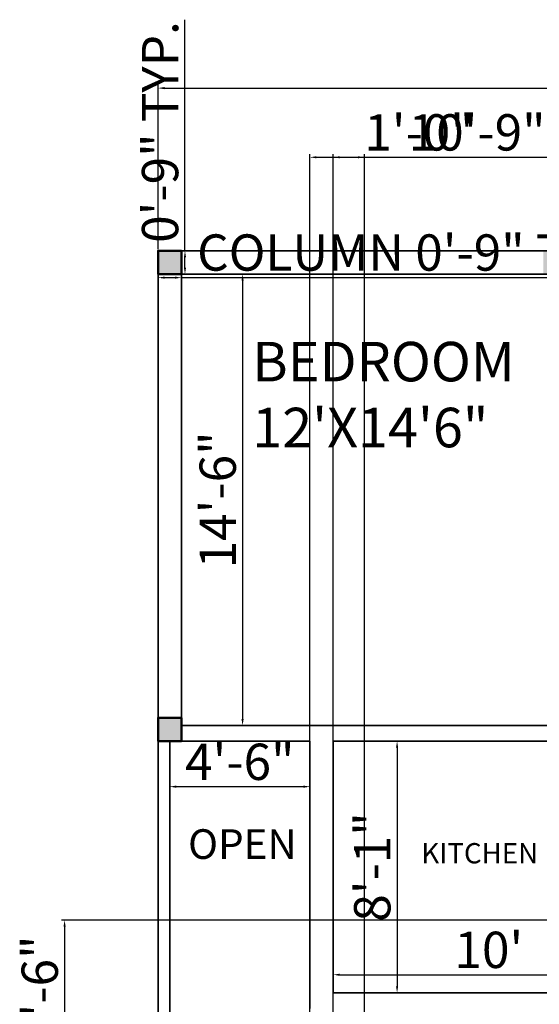
# Model space of a CAD drawing. Units: inches. Extents: x 3316 to 4157, y 2203 to 2977.
# Tile 2 of 4: x 3316 to 3517, y 2597 to 2977. Entities that reach past the tile are written whole.
import ezdxf

# ---------------------------------------------------------------- set-up
doc = ezdxf.new("R2010")
doc.units = ezdxf.units.IN
for name, color, linetype, lineweight in [('A-ANNO-DIMS', 2, 'Continuous', 18), ('A-AREA-IDEN', 7, 'Continuous', 25), ('A-COLS', 7, 'Continuous', 50), ('A-COLS-PATT', 4, 'Continuous', 13), ('A-WALL', 7, 'Continuous', 35), ('C-PROP', 7, 'Continuous', 35)]:
    doc.layers.add(name, color=color, linetype=linetype, lineweight=lineweight)
doc.styles.get("Standard").update_dxf_attribs({"font": 'arial.ttf'})
doc.dimstyles.new('ISO-25', dxfattribs={"dimtxt": 14, "dimasz": 2.5, "dimexe": 1.25, "dimexo": 0.625, "dimtad": 1, "dimlunit": 3, "dimtxsty": 'Standard', "dimcen": 2.5, "dimadec": 0, "dimazin": 0, "dimtfac": 1, "dimtmove": 0, "dimatfit": 3, "dimfxl": 1, "dimarcsym": 0})

# ---------------------------------------------------------------- blocks, each defined once
blk = doc.blocks.new('*D3')
at = {"layer": 'A-ANNO-DIMS', "color": 0, "lineweight": -2, "transparency": 16777216}
for p, q in [((3402.76, 2878.84), (3403.39, 2878.84)), ((3402.14, 2876.34), (3402.14, 2707.34)), ((3402.76, 2704.84), (3403.39, 2704.84))]:
    blk.add_line(p, q, dxfattribs=at)
at = {"layer": 'A-ANNO-DIMS', "color": 0, "transparency": 16777216}
for points in [[(3401.72, 2876.34), (3402.55, 2876.34), (3402.14, 2878.84)], [(3401.72, 2707.34), (3402.55, 2707.34), (3402.14, 2704.84)]]:
    blk.add_solid(points, dxfattribs=at)
at = {"layer": 'Defpoints', "color": 0, "transparency": 16777216}
for p in [(3402.14, 2878.84), (3402.14, 2704.84), (3402.14, 2704.84)]:
    blk.add_point(p, dxfattribs=at)
at = {"layer": 'A-ANNO-DIMS', "color": 0, "transparency": 16777216, "insert": (3394.37, 2791.84), "char_height": 14, "attachment_point": 5, "rotation": 90}
blk.add_mtext('14\'-6"', dxfattribs=at)
blk = doc.blocks.new('*D6')
at = {"layer": 'A-ANNO-DIMS', "color": 0, "lineweight": -2, "transparency": 16777216}
for p, q in [((3369.58, 2888.47), (3369.58, 2951.81)), ((3372.08, 2950.56), (3847.08, 2950.56)), ((3849.58, 2888.47), (3849.58, 2951.81))]:
    blk.add_line(p, q, dxfattribs=at)
at = {"layer": 'A-ANNO-DIMS', "color": 0, "transparency": 16777216}
for points in [[(3372.08, 2950.98), (3372.08, 2950.14), (3369.58, 2950.56)], [(3847.08, 2950.98), (3847.08, 2950.14), (3849.58, 2950.56)]]:
    blk.add_solid(points, dxfattribs=at)
at = {"layer": 'Defpoints', "color": 0, "transparency": 16777216}
for p in [(3849.58, 2950.56), (3369.58, 2887.84), (3849.58, 2887.84)]:
    blk.add_point(p, dxfattribs=at)
at = {"layer": 'A-ANNO-DIMS', "color": 0, "transparency": 16777216, "insert": (3609.58, 2958.33), "char_height": 14, "attachment_point": 5}
blk.add_mtext("40'", dxfattribs=at)
blk = doc.blocks.new('*D11')
at = {"layer": 'A-ANNO-DIMS', "color": 0, "lineweight": -2, "transparency": 16777216}
for p, q in [((3374.08, 2698.22), (3374.08, 2680.04)), ((3428.08, 2698.22), (3428.08, 2680.04)), ((3376.58, 2681.29), (3425.58, 2681.29))]:
    blk.add_line(p, q, dxfattribs=at)
at = {"layer": 'A-ANNO-DIMS', "color": 0, "transparency": 16777216}
for points in [[(3376.58, 2681.71), (3376.58, 2680.87), (3374.08, 2681.29)], [(3425.58, 2681.71), (3425.58, 2680.87), (3428.08, 2681.29)]]:
    blk.add_solid(points, dxfattribs=at)
at = {"layer": 'Defpoints', "color": 0, "transparency": 16777216}
for p in [(3374.08, 2698.84), (3428.08, 2698.84), (3428.08, 2681.29)]:
    blk.add_point(p, dxfattribs=at)
at = {"layer": 'A-ANNO-DIMS', "color": 0, "transparency": 16777216, "insert": (3401.08, 2689.06), "char_height": 14, "attachment_point": 5}
blk.add_mtext('4\'-6"', dxfattribs=at)
blk = doc.blocks.new('*D14')
at = {"layer": 'A-ANNO-DIMS', "color": 0, "lineweight": -2, "transparency": 16777216}
for p, q in [((3437.71, 2698.84), (3462.96, 2698.84)), ((3461.71, 2696.34), (3461.71, 2604.34)), ((3437.71, 2601.84), (3462.96, 2601.84))]:
    blk.add_line(p, q, dxfattribs=at)
at = {"layer": 'A-ANNO-DIMS', "color": 0, "transparency": 16777216}
for points in [[(3461.29, 2696.34), (3462.12, 2696.34), (3461.71, 2698.84)], [(3461.29, 2604.34), (3462.12, 2604.34), (3461.71, 2601.84)]]:
    blk.add_solid(points, dxfattribs=at)
at = {"layer": 'Defpoints', "color": 0, "transparency": 16777216}
for p in [(3437.08, 2698.84), (3437.08, 2601.84), (3461.71, 2601.84)]:
    blk.add_point(p, dxfattribs=at)
at = {"layer": 'A-ANNO-DIMS', "color": 0, "transparency": 16777216, "insert": (3453.94, 2650.34), "char_height": 14, "attachment_point": 5, "rotation": 90}
blk.add_mtext('8\'-1"', dxfattribs=at)
blk = doc.blocks.new('*D15')
at = {"layer": 'A-ANNO-DIMS', "color": 0, "lineweight": -2, "transparency": 16777216}
for p, q in [((3437.08, 2602.47), (3437.08, 2610.05)), ((3439.58, 2608.8), (3554.58, 2608.8)), ((3557.08, 2602.47), (3557.08, 2610.05))]:
    blk.add_line(p, q, dxfattribs=at)
at = {"layer": 'A-ANNO-DIMS', "color": 0, "transparency": 16777216}
for points in [[(3439.58, 2609.21), (3439.58, 2608.38), (3437.08, 2608.8)], [(3554.58, 2609.21), (3554.58, 2608.38), (3557.08, 2608.8)]]:
    blk.add_solid(points, dxfattribs=at)
at = {"layer": 'Defpoints', "color": 0, "transparency": 16777216}
for p in [(3557.08, 2608.8), (3437.08, 2601.84), (3557.08, 2601.84)]:
    blk.add_point(p, dxfattribs=at)
at = {"layer": 'A-ANNO-DIMS', "color": 0, "transparency": 16777216, "insert": (3497.08, 2616.57), "char_height": 14, "attachment_point": 5}
blk.add_mtext("10'", dxfattribs=at)
blk = doc.blocks.new('COL-9IN-SQ-PL')
blk.add_lwpolyline([(0, 0), (9, 0), (9, 9), (0, 9)], close=True)
blk = doc.blocks.new('*D36')
at = {"layer": 'A-ANNO-DIMS', "color": 0, "lineweight": -2, "transparency": 16777216}
for p, q in [((3369.58, 2878.22), (3369.58, 2876.24)), ((3372.08, 2877.49), (3376.08, 2877.49)), ((3378.58, 2878.22), (3378.58, 2876.24)), ((3378.58, 2877.49), (3557.7, 2877.49))]:
    blk.add_line(p, q, dxfattribs=at)
at = {"layer": 'A-ANNO-DIMS', "color": 0, "transparency": 16777216}
for points in [[(3372.08, 2877.91), (3372.08, 2877.08), (3369.58, 2877.49)], [(3376.08, 2877.91), (3376.08, 2877.08), (3378.58, 2877.49)]]:
    blk.add_solid(points, dxfattribs=at)
at = {"layer": 'Defpoints', "color": 0, "transparency": 16777216}
for p in [(3369.58, 2878.84), (3378.58, 2878.84), (3378.58, 2877.49)]:
    blk.add_point(p, dxfattribs=at)
at = {"layer": 'A-ANNO-DIMS', "color": 0, "transparency": 16777216, "insert": (3469.39, 2885.36), "char_height": 14, "attachment_point": 5}
blk.add_mtext('COLUMN 0\'-9" TYP.', dxfattribs=at)
blk = doc.blocks.new('*D37')
at = {"layer": 'A-ANNO-DIMS', "color": 0, "lineweight": -2, "transparency": 16777216}
for p, q in [((3379.93, 2887.84), (3379.93, 2976.93)), ((3379.21, 2887.84), (3381.18, 2887.84)), ((3379.93, 2881.34), (3379.93, 2885.34)), ((3379.21, 2878.84), (3381.18, 2878.84))]:
    blk.add_line(p, q, dxfattribs=at)
at = {"layer": 'A-ANNO-DIMS', "color": 0, "transparency": 16777216}
for points in [[(3379.52, 2885.34), (3380.35, 2885.34), (3379.93, 2887.84)], [(3379.52, 2881.34), (3380.35, 2881.34), (3379.93, 2878.84)]]:
    blk.add_solid(points, dxfattribs=at)
at = {"layer": 'Defpoints', "color": 0, "transparency": 16777216}
for p in [(3378.58, 2887.84), (3379.93, 2887.84), (3378.58, 2878.84)]:
    blk.add_point(p, dxfattribs=at)
at = {"layer": 'A-ANNO-DIMS', "color": 0, "transparency": 16777216, "insert": (3372.16, 2933.64), "char_height": 14, "attachment_point": 5, "rotation": 90}
blk.add_mtext('0\'-9" TYP.', dxfattribs=at)
blk = doc.blocks.new('*D50')
at = {"layer": 'A-ANNO-DIMS', "color": 0, "lineweight": -2, "transparency": 16777216}
for p, q in [((3751.46, 2629.84), (3332.28, 2629.84)), ((3333.53, 2627.34), (3333.53, 2578.34)), ((3751.46, 2575.84), (3332.28, 2575.84))]:
    blk.add_line(p, q, dxfattribs=at)
at = {"layer": 'A-ANNO-DIMS', "color": 0, "transparency": 16777216}
for points in [[(3333.12, 2627.34), (3333.95, 2627.34), (3333.53, 2629.84)], [(3333.12, 2578.34), (3333.95, 2578.34), (3333.53, 2575.84)]]:
    blk.add_solid(points, dxfattribs=at)
at = {"layer": 'Defpoints', "color": 0, "transparency": 16777216}
for p in [(3752.08, 2629.84), (3333.53, 2575.84), (3752.08, 2575.84)]:
    blk.add_point(p, dxfattribs=at)
at = {"layer": 'A-ANNO-DIMS', "color": 0, "transparency": 16777216, "insert": (3325.76, 2602.84), "char_height": 14, "attachment_point": 5, "rotation": 90}
blk.add_mtext('4\'-6"', dxfattribs=at)
blk = doc.blocks.new('*D59')
at = {"layer": 'A-ANNO-DIMS', "color": 0, "lineweight": -2, "transparency": 16777216}
for p, q in [((3437.08, 2544.97), (3437.08, 2925.14)), ((3439.58, 2923.89), (3446.58, 2923.89)), ((3449.08, 2544.97), (3449.08, 2925.14)), ((3449.08, 2923.89), (3488.73, 2923.89))]:
    blk.add_line(p, q, dxfattribs=at)
at = {"layer": 'A-ANNO-DIMS', "color": 0, "transparency": 16777216}
for points in [[(3439.58, 2924.31), (3439.58, 2923.48), (3437.08, 2923.89)], [(3446.58, 2924.31), (3446.58, 2923.48), (3449.08, 2923.89)]]:
    blk.add_solid(points, dxfattribs=at)
at = {"layer": 'Defpoints', "color": 0, "transparency": 16777216}
for p in [(3449.08, 2923.89), (3437.08, 2544.34), (3449.08, 2544.34)]:
    blk.add_point(p, dxfattribs=at)
at = {"layer": 'A-ANNO-DIMS', "color": 0, "transparency": 16777216, "insert": (3470.16, 2931.67), "char_height": 14, "attachment_point": 5}
blk.add_mtext('1\'-0"', dxfattribs=at)
blk = doc.blocks.new('*D60')
at = {"layer": 'A-ANNO-DIMS', "color": 0, "lineweight": -2, "transparency": 16777216}
for p, q in [((3428.08, 2544.97), (3428.08, 2925.14)), ((3430.58, 2923.89), (3554.58, 2923.89)), ((3557.08, 2544.97), (3557.08, 2925.14))]:
    blk.add_line(p, q, dxfattribs=at)
at = {"layer": 'A-ANNO-DIMS', "color": 0, "transparency": 16777216}
for points in [[(3430.58, 2924.31), (3430.58, 2923.48), (3428.08, 2923.89)], [(3554.58, 2924.31), (3554.58, 2923.48), (3557.08, 2923.89)]]:
    blk.add_solid(points, dxfattribs=at)
at = {"layer": 'Defpoints', "color": 0, "transparency": 16777216}
for p in [(3557.08, 2923.89), (3428.08, 2544.34), (3557.08, 2544.34)]:
    blk.add_point(p, dxfattribs=at)
at = {"layer": 'A-ANNO-DIMS', "color": 0, "transparency": 16777216, "insert": (3492.58, 2931.67), "char_height": 14, "attachment_point": 5}
blk.add_mtext('10\'-9"', dxfattribs=at)

msp = doc.modelspace()

# ---------------------------------------------------------------- hatches: boundary and pattern name
at = {"layer": 'A-COLS-PATT'}
h = msp.add_hatch(color=256, dxfattribs=at)
h.dxf.hatch_style = 1
h.paths.add_polyline_path([(3849.584, 2887.842), (3840.584, 2887.842), (3840.584, 2878.842), (3849.584, 2878.842)])
h.paths.add_polyline_path([(3696.584, 2887.842), (3687.584, 2887.842), (3687.584, 2878.842), (3696.584, 2878.842)])
h.paths.add_polyline_path([(3527.084, 2887.842), (3518.084, 2887.842), (3518.084, 2878.842), (3527.084, 2878.842)])
h.paths.add_polyline_path([(3378.584, 2887.842), (3369.584, 2887.842), (3369.584, 2878.842), (3378.584, 2878.842)])
h.paths.add_polyline_path([(3378.584, 2707.842), (3369.584, 2707.842), (3369.584, 2698.842), (3378.584, 2698.842)])
h.paths.add_polyline_path([(3561.584, 2704.842), (3552.584, 2704.842), (3552.584, 2695.842), (3561.584, 2695.842)])
h.paths.add_polyline_path([(3701.03, 2704.842), (3692.084, 2704.842), (3692.084, 2700.342), (3701.03, 2700.342)])
h.paths.add_polyline_path([(3701.03, 2700.342), (3692.03, 2700.342), (3692.03, 2695.842), (3701.03, 2695.842)])
h.paths.add_polyline_path([(3849.584, 2704.835), (3840.584, 2704.835), (3840.584, 2695.835), (3849.584, 2695.835)])
h.paths.add_polyline_path([(3378.584, 2505.342), (3369.584, 2505.342), (3369.584, 2496.342), (3378.584, 2496.342)])
h.paths.add_polyline_path([(3378.584, 2357.104), (3369.584, 2357.104), (3369.584, 2348.104), (3378.584, 2348.104)])
h.paths.add_polyline_path([(3512.084, 2505.342), (3503.084, 2505.342), (3503.084, 2496.342), (3512.084, 2496.342)])
h.paths.add_polyline_path([(3512.084, 2356.842), (3503.084, 2356.842), (3503.084, 2347.842), (3512.084, 2347.842)])
h.paths.add_polyline_path([(3701.115, 2505.342), (3696.584, 2505.342), (3696.584, 2500.842), (3696.584, 2496.342), (3701.115, 2496.342)])
h.paths.add_polyline_path([(3696.584, 2505.342), (3692.115, 2505.342), (3692.115, 2496.342), (3696.584, 2496.342), (3696.584, 2500.842)])
h.paths.add_polyline_path([(3699.422, 2356.842), (3690.422, 2356.842), (3690.422, 2347.842), (3699.422, 2347.842)])
h.paths.add_polyline_path([(3849.584, 2356.899), (3840.584, 2356.899), (3840.584, 2347.899), (3849.584, 2347.899)])
h.paths.add_polyline_path([(3849.584, 2505.307), (3840.584, 2505.307), (3840.584, 2496.307), (3849.584, 2496.307)])

# ---------------------------------------------------------------- linework, layer by layer
at = {"layer": 'A-WALL'}
for p, q in [((3378.584, 2878.842), (3378.584, 2704.842)), ((3369.584, 2704.842), (3369.584, 2700.342)), ((3378.584, 2704.842), (3561.584, 2704.842)), ((3378.584, 2698.842), (3374.084, 2698.842)), ((3374.084, 2505.342), (3374.084, 2698.842)), ((3378.584, 2698.842), (3428.084, 2698.842)), ((3428.084, 2698.842), (3428.084, 2601.842)), ((3437.084, 2700.342), (3437.084, 2700.342)), ((3437.084, 2698.842), (3437.084, 2672.702)), ((3437.084, 2698.842), (3552.584, 2698.842)), ((3437.084, 2601.842), (3437.084, 2672.702)), ((3428.084, 2601.842), (3428.084, 2595.842)), ((3557.084, 2601.842), (3437.084, 2601.842))]:
    msp.add_line(p, q, dxfattribs=at)
msp.add_lwpolyline([(3840.584, 2704.842), (3840.584, 2878.842), (3378.584, 2878.842), (3378.584, 2704.842)], dxfattribs=at)
at = {"layer": 'C-PROP'}
msp.add_lwpolyline([(3369.584, 2251.842), (3849.584, 2251.842), (3849.584, 2887.842), (3369.584, 2887.842)], close=True, dxfattribs=at)

# ---------------------------------------------------------------- block references
at = {"layer": 'A-COLS'}
for p in [(3369.584, 2878.842), (3369.584, 2698.842)]:
    msp.add_blockref('COL-9IN-SQ-PL', p, dxfattribs=at)

# ---------------------------------------------------------------- texts
at = {"layer": 'A-AREA-IDEN', "attachment_point": 1}
for s, width, gutter_width, insert, char_height in [('BEDROOM\\P12\'X14\'6"', 60.0775, 76.202, (3405.888, 2852.751), 15.2404), ('OPEN', 2.48803, 57.111, (3381.128, 2664.871), 11.4222), ('KITCHEN', 9.08392, 39.114, (3471.06, 2659.54), 7.8227)]:
    msp.add_mtext_dynamic_manual_height_columns(s, width=width, gutter_width=gutter_width, heights=[0], dxfattribs=dict(at, insert=insert, char_height=char_height))

# ---------------------------------------------------------------- dimensions: what is measured, and where the dimension line sits
at = {"layer": 'A-ANNO-DIMS'}
dim = msp.add_linear_dim(base=(3379.934, 2887.842), p1=(3378.584, 2878.842), p2=(3378.584, 2887.842), angle=90, text='<> TYP.', dimstyle='ISO-25', override={"dimdec": 1, "dimlfac": 1, "dimrnd": 0, "dimzin": 1, "dimdsep": 46, "dimlunit": 4, "dimfrac": 2}, dxfattribs=at)
dim.commit()
dim.dimension.update_dxf_attribs({"geometry": '*D37', "text_midpoint": (3372.161, 2933.636)})
for base, p1, p2, override, picture, middle in [((3849.584, 2950.561), (3369.584, 2887.842), (3849.584, 2887.842), {"dimclrd": 0, "dimclre": 0, "dimclrt": 0}, '*D6', (3609.584, 2958.334)), ((3557.084, 2923.892), (3428.084, 2544.342), (3557.084, 2544.342), {"dimdec": 1, "dimlfac": 1, "dimrnd": 0, "dimzin": 1, "dimdsep": 46, "dimlunit": 4, "dimfrac": 2}, '*D60', (3492.584, 2931.665)), ((3449.084, 2923.892), (3437.084, 2544.342), (3449.084, 2544.342), {"dimdec": 1, "dimlfac": 1, "dimrnd": 0, "dimzin": 1, "dimdsep": 46, "dimlunit": 4, "dimfrac": 2}, '*D59', (3470.158, 2931.665)), ((3428.084, 2681.29), (3374.084, 2698.842), (3428.084, 2698.842), {"dimclrd": 0, "dimclre": 0, "dimclrt": 0}, '*D11', (3401.084, 2689.063)), ((3557.084, 2608.797), (3437.084, 2601.842), (3557.084, 2601.842), {"dimclrd": 0, "dimclre": 0, "dimclrt": 0}, '*D15', (3497.084, 2616.57))]:
    dim = msp.add_linear_dim(base=base, p1=p1, p2=p2, dimstyle='ISO-25', override=override, dxfattribs=at)
    dim.commit()
    dim.dimension.update_dxf_attribs({"geometry": picture, "text_midpoint": middle})
dim = msp.add_linear_dim(base=(3378.584, 2877.492), p1=(3369.584, 2878.842), p2=(3378.584, 2878.842), text='COLUMN <> TYP.', dimstyle='ISO-25', override={"dimdec": 1, "dimlfac": 1, "dimrnd": 0, "dimzin": 1, "dimdsep": 46, "dimlunit": 4, "dimfrac": 2}, dxfattribs=at)
dim.commit()
dim.dimension.update_dxf_attribs({"geometry": '*D36', "text_midpoint": (3469.39, 2885.361)})
for base, p1, p2, angle, override, picture, middle in [((3402.138, 2704.842), (3402.138, 2878.842), (3402.138, 2704.842), 270, {"dimclrd": 0, "dimclre": 0, "dimclrt": 0}, '*D3', (3394.365, 2791.842)), ((3461.708, 2601.842), (3437.084, 2698.842), (3437.084, 2601.842), 90, {"dimclrd": 0, "dimclre": 0, "dimclrt": 0}, '*D14', (3453.935, 2650.342)), ((3333.534, 2575.842), (3752.084, 2629.842), (3752.084, 2575.842), 90, {"dimdec": 1, "dimlfac": 1, "dimrnd": 0, "dimzin": 1, "dimdsep": 46, "dimlunit": 4, "dimfrac": 2}, '*D50', (3325.761, 2602.842))]:
    dim = msp.add_linear_dim(base=base, p1=p1, p2=p2, angle=angle, dimstyle='ISO-25', override=override, dxfattribs=at)
    dim.commit()
    dim.dimension.update_dxf_attribs({"geometry": picture, "text_midpoint": middle})

doc.saveas('drawing.dxf')
